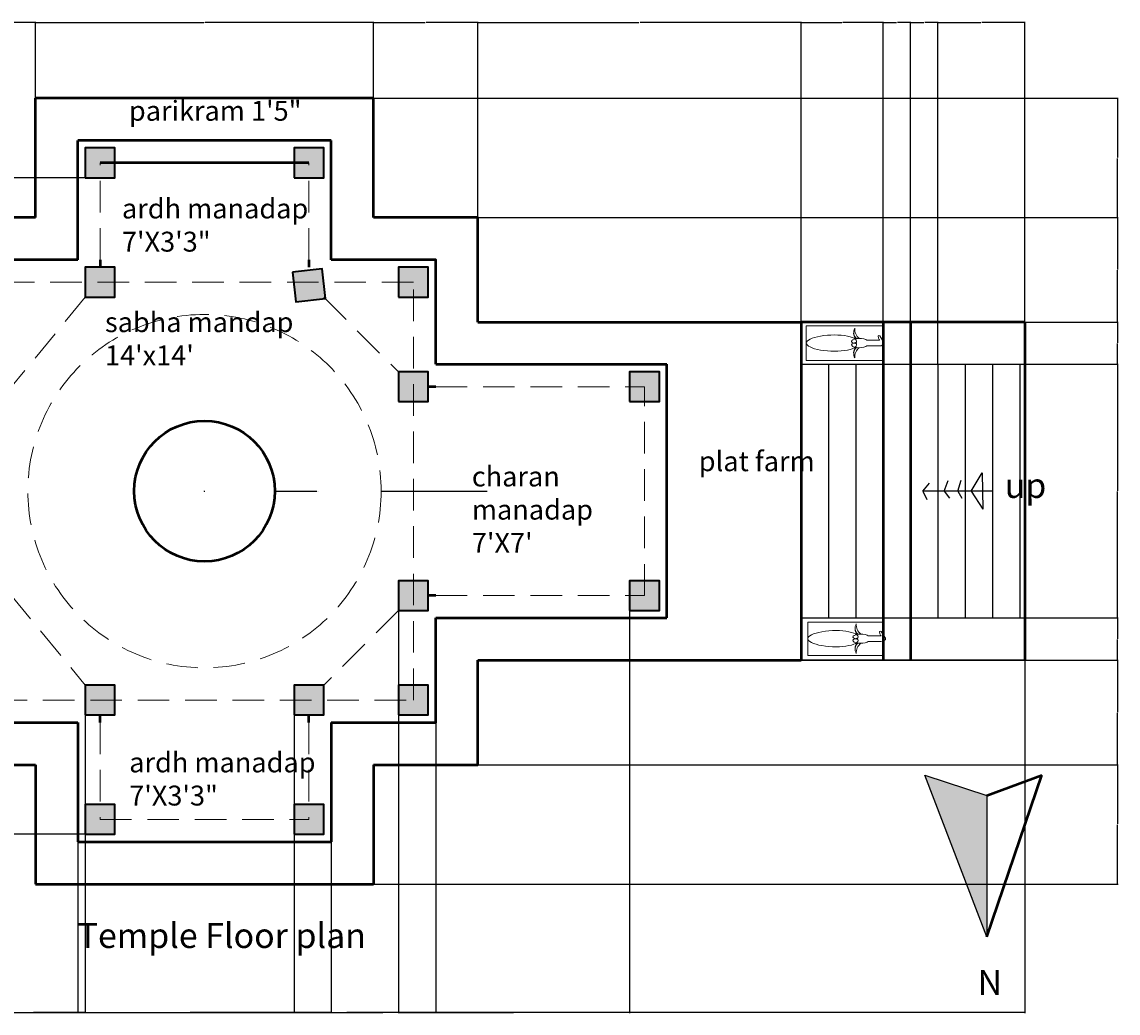
# Model space of a CAD drawing. Units: inches. Extents: x 386 to 107067, y -7 to 96314.
# Tile 6 of 10: x 766 to 1206, y 872 to 1271. Entities that reach past the tile are written whole.
import ezdxf

# ---------------------------------------------------------------- set-up
doc = ezdxf.new("R2010")
doc.units = ezdxf.units.IN
doc.linetypes.add('DASHED', pattern=[19.05, 12.7, -6.35])
for name, color, linetype, lineweight in [('A-ANNO-DIMS', 2, 'Continuous', 18), ('A-ANNO-SYMB', 2, 'Continuous', 25), ('A-ANNO-TEXT', 7, 'Continuous', 25), ('A-AREA-IDEN', 3, 'Continuous', 18), ('A-COLS', 1, 'Continuous', 35), ('A-FLOR-OVHD', 8, 'DASHED', 18), ('A-FLOR-STRS', 3, 'Continuous', 25), ('A-FURN', 8, 'Continuous', 18), ('A-WALL', 7, 'Continuous', 50)]:
    doc.layers.add(name, color=color, linetype=linetype, lineweight=lineweight)
doc.styles.get("Standard").update_dxf_attribs({"font": 'arial.ttf'})
doc.dimstyles.get("Standard").update_dxf_attribs({"dimtxt": 0.18, "dimasz": 0.18, "dimexe": 0.18, "dimexo": 0.0625, "dimgap": 0.09, "dimtad": 0, "dimtih": 1, "dimtoh": 1, "dimdec": 4, "dimzin": 0, "dimdsep": 46, "dimtxsty": 'Standard', "dimcen": 0.09, "dimadec": 0, "dimazin": 0, "dimtfac": 1, "dimtdec": 4, "dimtofl": 0, "dimtmove": 0, "dimatfit": 3, "dimfxl": 1, "dimtolj": 1, "dimtzin": 0, "dimarcsym": 0})

# ---------------------------------------------------------------- blocks, each defined once
blk = doc.blocks.new('COL-300')
h = blk.add_hatch(color=256)
h.dxf.hatch_style = 1
h.paths.add_polyline_path([(761.03, 1172.09), (749.03, 1172.09), (749.03, 1160.09), (761.03, 1160.09)])
blk.add_lwpolyline([(749.03, 1160.09), (761.03, 1160.09), (761.03, 1172.09), (749.03, 1172.09)], close=True)
blk = doc.blocks.new('*D8')
at = {"layer": 'A-ANNO-DIMS', "color": 0, "lineweight": -2, "transparency": 16777216}
for p, q in [((623.03, 1046.53), (623.03, 872.22)), ((1169.03, 1014.03), (1169.03, 872.22)), ((623.21, 872.4), (895.74, 872.4)), ((1168.85, 872.4), (896.31, 872.4))]:
    blk.add_line(p, q, dxfattribs=at)
at = {"layer": 'A-ANNO-DIMS', "color": 0, "transparency": 16777216}
for points in [[(623.21, 872.43), (623.21, 872.37), (623.03, 872.4)], [(1168.85, 872.43), (1168.85, 872.37), (1169.03, 872.4)]]:
    blk.add_solid(points, dxfattribs=at)
at = {"layer": 'Defpoints', "color": 0, "transparency": 16777216}
for p in [(623.03, 1046.59), (1169.03, 1014.09), (1169.03, 872.4)]:
    blk.add_point(p, dxfattribs=at)
at = {"layer": 'A-ANNO-DIMS', "color": 0, "transparency": 16777216, "insert": (896.03, 872.4), "char_height": 0.18, "attachment_point": 5}
blk.add_mtext('\\A1;546', dxfattribs=at)
blk = doc.blocks.new('*D10')
at = {"layer": 'A-ANNO-DIMS', "color": 0, "lineweight": -2, "transparency": 16777216}
for p, q in [((729.03, 1192.15), (729.03, 1270.77)), ((729.21, 1270.59), (749.8, 1270.59)), ((770.85, 1270.59), (750.25, 1270.59)), ((771.03, 1240.15), (771.03, 1270.77))]:
    blk.add_line(p, q, dxfattribs=at)
at = {"layer": 'A-ANNO-DIMS', "color": 0, "transparency": 16777216}
for points in [[(729.21, 1270.62), (729.21, 1270.56), (729.03, 1270.59)], [(770.85, 1270.62), (770.85, 1270.56), (771.03, 1270.59)]]:
    blk.add_solid(points, dxfattribs=at)
at = {"layer": 'Defpoints', "color": 0, "transparency": 16777216}
for p in [(771.03, 1270.59), (771.03, 1240.09), (729.03, 1192.09)]:
    blk.add_point(p, dxfattribs=at)
at = {"layer": 'A-ANNO-DIMS', "color": 0, "transparency": 16777216, "insert": (750.03, 1270.59), "char_height": 0.18, "attachment_point": 5}
blk.add_mtext('\\A1;42', dxfattribs=at)
blk = doc.blocks.new('*D11')
at = {"layer": 'A-ANNO-DIMS', "color": 0, "lineweight": -2, "transparency": 16777216}
for p, q in [((771.03, 1240.15), (771.03, 1270.77)), ((771.21, 1270.59), (838.74, 1270.59)), ((906.85, 1270.59), (839.31, 1270.59)), ((907.03, 1240.15), (907.03, 1270.77))]:
    blk.add_line(p, q, dxfattribs=at)
at = {"layer": 'A-ANNO-DIMS', "color": 0, "transparency": 16777216}
for points in [[(771.21, 1270.62), (771.21, 1270.56), (771.03, 1270.59)], [(906.85, 1270.62), (906.85, 1270.56), (907.03, 1270.59)]]:
    blk.add_solid(points, dxfattribs=at)
at = {"layer": 'Defpoints', "color": 0, "transparency": 16777216}
for p in [(907.03, 1270.59), (771.03, 1240.09), (907.03, 1240.09)]:
    blk.add_point(p, dxfattribs=at)
at = {"layer": 'A-ANNO-DIMS', "color": 0, "transparency": 16777216, "insert": (839.03, 1270.59), "char_height": 0.18, "attachment_point": 5}
blk.add_mtext('\\A1;136', dxfattribs=at)
blk = doc.blocks.new('*D12')
at = {"layer": 'A-ANNO-DIMS', "color": 0, "lineweight": -2, "transparency": 16777216}
for p, q in [((907.03, 1240.15), (907.03, 1270.77)), ((907.21, 1270.59), (927.8, 1270.59)), ((948.85, 1270.59), (928.25, 1270.59)), ((949.03, 1192.15), (949.03, 1270.77))]:
    blk.add_line(p, q, dxfattribs=at)
at = {"layer": 'A-ANNO-DIMS', "color": 0, "transparency": 16777216}
for points in [[(907.21, 1270.62), (907.21, 1270.56), (907.03, 1270.59)], [(948.85, 1270.62), (948.85, 1270.56), (949.03, 1270.59)]]:
    blk.add_solid(points, dxfattribs=at)
at = {"layer": 'Defpoints', "color": 0, "transparency": 16777216}
for p in [(949.03, 1270.59), (907.03, 1240.09), (949.03, 1192.09)]:
    blk.add_point(p, dxfattribs=at)
at = {"layer": 'A-ANNO-DIMS', "color": 0, "transparency": 16777216, "insert": (928.03, 1270.59), "char_height": 0.18, "attachment_point": 5}
blk.add_mtext('\\A1;42', dxfattribs=at)
blk = doc.blocks.new('*D13')
at = {"layer": 'A-ANNO-DIMS', "color": 0, "lineweight": -2, "transparency": 16777216}
for p, q in [((949.03, 1150.15), (949.03, 1270.77)), ((949.21, 1270.59), (1013.75, 1270.59)), ((1078.85, 1270.59), (1014.31, 1270.59)), ((1079.03, 1150.15), (1079.03, 1270.77))]:
    blk.add_line(p, q, dxfattribs=at)
at = {"layer": 'A-ANNO-DIMS', "color": 0, "transparency": 16777216}
for points in [[(949.21, 1270.62), (949.21, 1270.56), (949.03, 1270.59)], [(1078.85, 1270.62), (1078.85, 1270.56), (1079.03, 1270.59)]]:
    blk.add_solid(points, dxfattribs=at)
at = {"layer": 'Defpoints', "color": 0, "transparency": 16777216}
for p in [(1079.03, 1270.59), (949.03, 1150.09), (1079.03, 1150.09)]:
    blk.add_point(p, dxfattribs=at)
at = {"layer": 'A-ANNO-DIMS', "color": 0, "transparency": 16777216, "insert": (1014.03, 1270.59), "char_height": 0.18, "attachment_point": 5}
blk.add_mtext('\\A1;130', dxfattribs=at)
blk = doc.blocks.new('*D14')
at = {"layer": 'A-ANNO-DIMS', "color": 0, "lineweight": -2, "transparency": 16777216}
for p, q in [((1079.03, 1150.15), (1079.03, 1270.77)), ((1079.21, 1270.59), (1095.31, 1270.59)), ((1111.85, 1270.59), (1095.74, 1270.59)), ((1112.03, 1150.15), (1112.03, 1270.77))]:
    blk.add_line(p, q, dxfattribs=at)
at = {"layer": 'A-ANNO-DIMS', "color": 0, "transparency": 16777216}
for points in [[(1079.21, 1270.62), (1079.21, 1270.56), (1079.03, 1270.59)], [(1111.85, 1270.62), (1111.85, 1270.56), (1112.03, 1270.59)]]:
    blk.add_solid(points, dxfattribs=at)
at = {"layer": 'Defpoints', "color": 0, "transparency": 16777216}
for p in [(1112.03, 1270.59), (1079.03, 1150.09), (1112.03, 1150.09)]:
    blk.add_point(p, dxfattribs=at)
at = {"layer": 'A-ANNO-DIMS', "color": 0, "transparency": 16777216, "insert": (1095.53, 1270.59), "char_height": 0.18, "attachment_point": 5}
blk.add_mtext('\\A1;33', dxfattribs=at)
blk = doc.blocks.new('*D15')
at = {"layer": 'A-ANNO-DIMS', "color": 0, "lineweight": -2, "transparency": 16777216}
for p, q in [((1112.03, 1150.15), (1112.03, 1270.77)), ((1112.21, 1270.59), (1117.33, 1270.59)), ((1122.85, 1270.59), (1117.72, 1270.59)), ((1123.03, 1150.15), (1123.03, 1270.77))]:
    blk.add_line(p, q, dxfattribs=at)
at = {"layer": 'A-ANNO-DIMS', "color": 0, "transparency": 16777216}
for points in [[(1112.21, 1270.62), (1112.21, 1270.56), (1112.03, 1270.59)], [(1122.85, 1270.62), (1122.85, 1270.56), (1123.03, 1270.59)]]:
    blk.add_solid(points, dxfattribs=at)
at = {"layer": 'Defpoints', "color": 0, "transparency": 16777216}
for p in [(1123.03, 1270.59), (1112.03, 1150.09), (1123.03, 1150.09)]:
    blk.add_point(p, dxfattribs=at)
at = {"layer": 'A-ANNO-DIMS', "color": 0, "transparency": 16777216, "insert": (1117.53, 1270.59), "char_height": 0.18, "attachment_point": 5}
blk.add_mtext('\\A1;11', dxfattribs=at)
blk = doc.blocks.new('*D16')
at = {"layer": 'A-ANNO-DIMS', "color": 0, "lineweight": -2, "transparency": 16777216}
for p, q in [((1123.03, 1150.15), (1123.03, 1270.77)), ((1123.21, 1270.59), (1128.33, 1270.59)), ((1133.85, 1270.59), (1128.72, 1270.59)), ((1134.03, 1133.15), (1134.03, 1270.77))]:
    blk.add_line(p, q, dxfattribs=at)
at = {"layer": 'A-ANNO-DIMS', "color": 0, "transparency": 16777216}
for points in [[(1123.21, 1270.62), (1123.21, 1270.56), (1123.03, 1270.59)], [(1133.85, 1270.62), (1133.85, 1270.56), (1134.03, 1270.59)]]:
    blk.add_solid(points, dxfattribs=at)
at = {"layer": 'Defpoints', "color": 0, "transparency": 16777216}
for p in [(1134.03, 1270.59), (1123.03, 1150.09), (1134.03, 1133.09)]:
    blk.add_point(p, dxfattribs=at)
at = {"layer": 'A-ANNO-DIMS', "color": 0, "transparency": 16777216, "insert": (1128.53, 1270.59), "char_height": 0.18, "attachment_point": 5}
blk.add_mtext('\\A1;11', dxfattribs=at)
blk = doc.blocks.new('*D17')
at = {"layer": 'A-ANNO-DIMS', "color": 0, "lineweight": -2, "transparency": 16777216}
for p, q in [((1134.03, 1133.15), (1134.03, 1270.77)), ((1134.21, 1270.59), (1151.31, 1270.59)), ((1168.85, 1270.59), (1151.74, 1270.59)), ((1169.03, 1150.15), (1169.03, 1270.77))]:
    blk.add_line(p, q, dxfattribs=at)
at = {"layer": 'A-ANNO-DIMS', "color": 0, "transparency": 16777216}
for points in [[(1134.21, 1270.62), (1134.21, 1270.56), (1134.03, 1270.59)], [(1168.85, 1270.62), (1168.85, 1270.56), (1169.03, 1270.59)]]:
    blk.add_solid(points, dxfattribs=at)
at = {"layer": 'Defpoints', "color": 0, "transparency": 16777216}
for p in [(1169.03, 1270.59), (1169.03, 1150.09), (1134.03, 1133.09)]:
    blk.add_point(p, dxfattribs=at)
at = {"layer": 'A-ANNO-DIMS', "color": 0, "transparency": 16777216, "insert": (1151.53, 1270.59), "char_height": 0.18, "attachment_point": 5}
blk.add_mtext('\\A1;35', dxfattribs=at)
blk = doc.blocks.new('*D18')
at = {"layer": 'A-ANNO-DIMS', "color": 0, "lineweight": -2, "transparency": 16777216}
for p, q in [((949.09, 972.09), (1206.45, 972.09)), ((1206.27, 971.91), (1206.27, 948.27)), ((1206.27, 924.27), (1206.27, 947.91)), ((907.09, 924.09), (1206.45, 924.09))]:
    blk.add_line(p, q, dxfattribs=at)
at = {"layer": 'A-ANNO-DIMS', "color": 0, "transparency": 16777216}
for points in [[(1206.24, 971.91), (1206.3, 971.91), (1206.27, 972.09)], [(1206.24, 924.27), (1206.3, 924.27), (1206.27, 924.09)]]:
    blk.add_solid(points, dxfattribs=at)
at = {"layer": 'Defpoints', "color": 0, "transparency": 16777216}
for p in [(949.03, 972.09), (1206.27, 972.09), (907.03, 924.09)]:
    blk.add_point(p, dxfattribs=at)
at = {"layer": 'A-ANNO-DIMS', "color": 0, "transparency": 16777216, "insert": (1206.27, 948.09), "char_height": 0.18, "attachment_point": 5}
blk.add_mtext('\\A1;48', dxfattribs=at)
blk = doc.blocks.new('*D19')
at = {"layer": 'A-ANNO-DIMS', "color": 0, "lineweight": -2, "transparency": 16777216}
for p, q in [((1079.09, 1014.09), (1206.45, 1014.09)), ((1206.27, 1013.91), (1206.27, 993.27)), ((1206.27, 972.27), (1206.27, 992.91)), ((949.09, 972.09), (1206.45, 972.09))]:
    blk.add_line(p, q, dxfattribs=at)
at = {"layer": 'A-ANNO-DIMS', "color": 0, "transparency": 16777216}
for points in [[(1206.24, 1013.91), (1206.3, 1013.91), (1206.27, 1014.09)], [(1206.24, 972.27), (1206.3, 972.27), (1206.27, 972.09)]]:
    blk.add_solid(points, dxfattribs=at)
at = {"layer": 'Defpoints', "color": 0, "transparency": 16777216}
for p in [(1079.03, 1014.09), (1206.27, 1014.09), (949.03, 972.09)]:
    blk.add_point(p, dxfattribs=at)
at = {"layer": 'A-ANNO-DIMS', "color": 0, "transparency": 16777216, "insert": (1206.27, 993.09), "char_height": 0.18, "attachment_point": 5}
blk.add_mtext('\\A1;42', dxfattribs=at)
blk = doc.blocks.new('*D20')
at = {"layer": 'A-ANNO-DIMS', "color": 0, "lineweight": -2, "transparency": 16777216}
for p, q in [((1169.09, 1031.09), (1206.45, 1031.09)), ((1206.27, 1030.91), (1206.27, 1022.77)), ((1206.27, 1014.27), (1206.27, 1022.41)), ((1079.09, 1014.09), (1206.45, 1014.09))]:
    blk.add_line(p, q, dxfattribs=at)
at = {"layer": 'A-ANNO-DIMS', "color": 0, "transparency": 16777216}
for points in [[(1206.24, 1030.91), (1206.3, 1030.91), (1206.27, 1031.09)], [(1206.24, 1014.27), (1206.3, 1014.27), (1206.27, 1014.09)]]:
    blk.add_solid(points, dxfattribs=at)
at = {"layer": 'Defpoints', "color": 0, "transparency": 16777216}
for p in [(1169.03, 1031.09), (1206.27, 1031.09), (1079.03, 1014.09)]:
    blk.add_point(p, dxfattribs=at)
at = {"layer": 'A-ANNO-DIMS', "color": 0, "transparency": 16777216, "insert": (1206.27, 1022.59), "char_height": 0.18, "attachment_point": 5}
blk.add_mtext('\\A1;17', dxfattribs=at)
blk = doc.blocks.new('*D21')
at = {"layer": 'A-ANNO-DIMS', "color": 0, "lineweight": -2, "transparency": 16777216}
for p, q in [((1169.09, 1133.09), (1206.45, 1133.09)), ((1206.27, 1132.91), (1206.27, 1082.27)), ((1206.27, 1031.27), (1206.27, 1081.91)), ((1169.09, 1031.09), (1206.45, 1031.09))]:
    blk.add_line(p, q, dxfattribs=at)
at = {"layer": 'A-ANNO-DIMS', "color": 0, "transparency": 16777216}
for points in [[(1206.24, 1132.91), (1206.3, 1132.91), (1206.27, 1133.09)], [(1206.24, 1031.27), (1206.3, 1031.27), (1206.27, 1031.09)]]:
    blk.add_solid(points, dxfattribs=at)
at = {"layer": 'Defpoints', "color": 0, "transparency": 16777216}
for p in [(1169.03, 1133.09), (1206.27, 1133.09), (1169.03, 1031.09)]:
    blk.add_point(p, dxfattribs=at)
at = {"layer": 'A-ANNO-DIMS', "color": 0, "transparency": 16777216, "insert": (1206.27, 1082.09), "char_height": 0.18, "attachment_point": 5}
blk.add_mtext('\\A1;102', dxfattribs=at)
blk = doc.blocks.new('*D22')
at = {"layer": 'A-ANNO-DIMS', "color": 0, "lineweight": -2, "transparency": 16777216}
for p, q in [((1079.09, 1150.09), (1206.45, 1150.09)), ((1206.27, 1149.91), (1206.27, 1141.77)), ((1206.27, 1133.27), (1206.27, 1141.41)), ((1169.09, 1133.09), (1206.45, 1133.09))]:
    blk.add_line(p, q, dxfattribs=at)
at = {"layer": 'A-ANNO-DIMS', "color": 0, "transparency": 16777216}
for points in [[(1206.24, 1149.91), (1206.3, 1149.91), (1206.27, 1150.09)], [(1206.24, 1133.27), (1206.3, 1133.27), (1206.27, 1133.09)]]:
    blk.add_solid(points, dxfattribs=at)
at = {"layer": 'Defpoints', "color": 0, "transparency": 16777216}
for p in [(1079.03, 1150.09), (1206.27, 1150.09), (1169.03, 1133.09)]:
    blk.add_point(p, dxfattribs=at)
at = {"layer": 'A-ANNO-DIMS', "color": 0, "transparency": 16777216, "insert": (1206.27, 1141.59), "char_height": 0.18, "attachment_point": 5}
blk.add_mtext('\\A1;17', dxfattribs=at)
blk = doc.blocks.new('*D23')
at = {"layer": 'A-ANNO-DIMS', "color": 0, "lineweight": -2, "transparency": 16777216}
for p, q in [((949.09, 1192.09), (1206.45, 1192.09)), ((1206.27, 1191.91), (1206.27, 1171.27)), ((1206.27, 1150.27), (1206.27, 1170.91)), ((949.09, 1150.09), (1206.45, 1150.09))]:
    blk.add_line(p, q, dxfattribs=at)
at = {"layer": 'A-ANNO-DIMS', "color": 0, "transparency": 16777216}
for points in [[(1206.24, 1191.91), (1206.3, 1191.91), (1206.27, 1192.09)], [(1206.24, 1150.27), (1206.3, 1150.27), (1206.27, 1150.09)]]:
    blk.add_solid(points, dxfattribs=at)
at = {"layer": 'Defpoints', "color": 0, "transparency": 16777216}
for p in [(949.03, 1192.09), (1206.27, 1192.09), (949.03, 1150.09)]:
    blk.add_point(p, dxfattribs=at)
at = {"layer": 'A-ANNO-DIMS', "color": 0, "transparency": 16777216, "insert": (1206.27, 1171.09), "char_height": 0.18, "attachment_point": 5}
blk.add_mtext('\\A1;42', dxfattribs=at)
blk = doc.blocks.new('*D24')
at = {"layer": 'A-ANNO-DIMS', "color": 0, "lineweight": -2, "transparency": 16777216}
for p, q in [((907.09, 1240.09), (1206.45, 1240.09)), ((1206.27, 1239.91), (1206.27, 1216.27)), ((1206.27, 1192.27), (1206.27, 1215.91)), ((907.09, 1192.09), (1206.45, 1192.09))]:
    blk.add_line(p, q, dxfattribs=at)
at = {"layer": 'A-ANNO-DIMS', "color": 0, "transparency": 16777216}
for points in [[(1206.24, 1239.91), (1206.3, 1239.91), (1206.27, 1240.09)], [(1206.24, 1192.27), (1206.3, 1192.27), (1206.27, 1192.09)]]:
    blk.add_solid(points, dxfattribs=at)
at = {"layer": 'Defpoints', "color": 0, "transparency": 16777216}
for p in [(907.03, 1240.09), (1206.27, 1240.09), (907.03, 1192.09)]:
    blk.add_point(p, dxfattribs=at)
at = {"layer": 'A-ANNO-DIMS', "color": 0, "transparency": 16777216, "insert": (1206.27, 1216.09), "char_height": 0.18, "attachment_point": 5}
blk.add_mtext('\\A1;48', dxfattribs=at)
blk = doc.blocks.new('*D25')
at = {"layer": 'A-ANNO-DIMS', "color": 0, "lineweight": -2, "transparency": 16777216}
for p, q in [((788.03, 941.03), (788.03, 872.22)), ((890.03, 941.03), (890.03, 872.22)), ((788.21, 872.4), (838.75, 872.4)), ((889.85, 872.4), (839.3, 872.4))]:
    blk.add_line(p, q, dxfattribs=at)
at = {"layer": 'A-ANNO-DIMS', "color": 0, "transparency": 16777216}
for points in [[(788.21, 872.43), (788.21, 872.37), (788.03, 872.4)], [(889.85, 872.43), (889.85, 872.37), (890.03, 872.4)]]:
    blk.add_solid(points, dxfattribs=at)
at = {"layer": 'Defpoints', "color": 0, "transparency": 16777216}
for p in [(788.03, 941.09), (890.03, 941.09), (890.03, 872.4)]:
    blk.add_point(p, dxfattribs=at)
at = {"layer": 'A-ANNO-DIMS', "color": 0, "transparency": 16777216, "insert": (839.03, 872.4), "char_height": 0.18, "attachment_point": 5}
blk.add_mtext('\\A1;102', dxfattribs=at)
blk = doc.blocks.new('*D26')
at = {"layer": 'A-ANNO-DIMS', "color": 0, "lineweight": -2, "transparency": 16777216}
for p, q in [((932.03, 989.03), (932.03, 872.22)), ((890.03, 941.03), (890.03, 872.22)), ((890.21, 872.4), (910.8, 872.4)), ((931.85, 872.4), (911.25, 872.4))]:
    blk.add_line(p, q, dxfattribs=at)
at = {"layer": 'A-ANNO-DIMS', "color": 0, "transparency": 16777216}
for points in [[(890.21, 872.43), (890.21, 872.37), (890.03, 872.4)], [(931.85, 872.43), (931.85, 872.37), (932.03, 872.4)]]:
    blk.add_solid(points, dxfattribs=at)
at = {"layer": 'Defpoints', "color": 0, "transparency": 16777216}
for p in [(932.03, 989.09), (890.03, 941.09), (932.03, 872.4)]:
    blk.add_point(p, dxfattribs=at)
at = {"layer": 'A-ANNO-DIMS', "color": 0, "transparency": 16777216, "insert": (911.03, 872.4), "char_height": 0.18, "attachment_point": 5}
blk.add_mtext('\\A1;42', dxfattribs=at)
blk = doc.blocks.new('*D27')
at = {"layer": 'A-ANNO-DIMS', "color": 0, "lineweight": -2, "transparency": 16777216}
for p, q in [((749.03, 992.03), (749.03, 872.22)), ((791.03, 992.03), (791.03, 872.22)), ((749.21, 872.4), (769.8, 872.4)), ((790.85, 872.4), (770.25, 872.4))]:
    blk.add_line(p, q, dxfattribs=at)
at = {"layer": 'A-ANNO-DIMS', "color": 0, "transparency": 16777216}
for points in [[(749.21, 872.43), (749.21, 872.37), (749.03, 872.4)], [(790.85, 872.43), (790.85, 872.37), (791.03, 872.4)]]:
    blk.add_solid(points, dxfattribs=at)
at = {"layer": 'Defpoints', "color": 0, "transparency": 16777216}
for p in [(749.03, 992.09), (791.03, 992.09), (791.03, 872.4)]:
    blk.add_point(p, dxfattribs=at)
at = {"layer": 'A-ANNO-DIMS', "color": 0, "transparency": 16777216, "insert": (770.03, 872.4), "char_height": 0.18, "attachment_point": 5}
blk.add_mtext('\\A1;42', dxfattribs=at)
blk = doc.blocks.new('*D28')
at = {"layer": 'A-ANNO-DIMS', "color": 0, "lineweight": -2, "transparency": 16777216}
for p, q in [((791.03, 992.03), (791.03, 872.22)), ((875.03, 992.03), (875.03, 872.22)), ((791.21, 872.4), (832.81, 872.4)), ((874.85, 872.4), (833.24, 872.4))]:
    blk.add_line(p, q, dxfattribs=at)
at = {"layer": 'A-ANNO-DIMS', "color": 0, "transparency": 16777216}
for points in [[(791.21, 872.43), (791.21, 872.37), (791.03, 872.4)], [(874.85, 872.43), (874.85, 872.37), (875.03, 872.4)]]:
    blk.add_solid(points, dxfattribs=at)
at = {"layer": 'Defpoints', "color": 0, "transparency": 16777216}
for p in [(791.03, 992.09), (875.03, 992.09), (875.03, 872.4)]:
    blk.add_point(p, dxfattribs=at)
at = {"layer": 'A-ANNO-DIMS', "color": 0, "transparency": 16777216, "insert": (833.03, 872.4), "char_height": 0.18, "attachment_point": 5}
blk.add_mtext('\\A1;84', dxfattribs=at)
blk = doc.blocks.new('*D29')
at = {"layer": 'A-ANNO-DIMS', "color": 0, "lineweight": -2, "transparency": 16777216}
for p, q in [((875.03, 992.03), (875.03, 872.22)), ((917.03, 992.03), (917.03, 872.22)), ((875.21, 872.4), (895.8, 872.4)), ((916.85, 872.4), (896.25, 872.4))]:
    blk.add_line(p, q, dxfattribs=at)
at = {"layer": 'A-ANNO-DIMS', "color": 0, "transparency": 16777216}
for points in [[(875.21, 872.43), (875.21, 872.37), (875.03, 872.4)], [(916.85, 872.43), (916.85, 872.37), (917.03, 872.4)]]:
    blk.add_solid(points, dxfattribs=at)
at = {"layer": 'Defpoints', "color": 0, "transparency": 16777216}
for p in [(875.03, 992.09), (917.03, 992.09), (917.03, 872.4)]:
    blk.add_point(p, dxfattribs=at)
at = {"layer": 'A-ANNO-DIMS', "color": 0, "transparency": 16777216, "insert": (896.03, 872.4), "char_height": 0.18, "attachment_point": 5}
blk.add_mtext('\\A1;42', dxfattribs=at)
blk = doc.blocks.new('*D30')
at = {"layer": 'A-ANNO-DIMS', "color": 0, "lineweight": -2, "transparency": 16777216}
for p, q in [((917.03, 1034.03), (917.03, 872.22)), ((1010.03, 1034.03), (1010.03, 872.22)), ((917.21, 872.4), (963.31, 872.4)), ((1009.85, 872.4), (963.74, 872.4))]:
    blk.add_line(p, q, dxfattribs=at)
at = {"layer": 'A-ANNO-DIMS', "color": 0, "transparency": 16777216}
for points in [[(917.21, 872.43), (917.21, 872.37), (917.03, 872.4)], [(1009.85, 872.43), (1009.85, 872.37), (1010.03, 872.4)]]:
    blk.add_solid(points, dxfattribs=at)
at = {"layer": 'Defpoints', "color": 0, "transparency": 16777216}
for p in [(917.03, 1034.09), (1010.03, 1034.09), (1010.03, 872.4)]:
    blk.add_point(p, dxfattribs=at)
at = {"layer": 'A-ANNO-DIMS', "color": 0, "transparency": 16777216, "insert": (963.53, 872.4), "char_height": 0.18, "attachment_point": 5}
blk.add_mtext('\\A1;93', dxfattribs=at)
blk = doc.blocks.new('*D31')
at = {"layer": 'A-ANNO-DIMS', "color": 0, "lineweight": -2, "transparency": 16777216}
for p, q in [((748.96, 992.09), (592.35, 992.09)), ((592.53, 991.91), (592.53, 968.27)), ((592.53, 944.27), (592.53, 967.91)), ((790.96, 944.09), (592.35, 944.09))]:
    blk.add_line(p, q, dxfattribs=at)
at = {"layer": 'A-ANNO-DIMS', "color": 0, "transparency": 16777216}
for points in [[(592.5, 991.91), (592.56, 991.91), (592.53, 992.09)], [(592.5, 944.27), (592.56, 944.27), (592.53, 944.09)]]:
    blk.add_solid(points, dxfattribs=at)
at = {"layer": 'Defpoints', "color": 0, "transparency": 16777216}
for p in [(592.53, 992.09), (749.03, 992.09), (791.03, 944.09)]:
    blk.add_point(p, dxfattribs=at)
at = {"layer": 'A-ANNO-DIMS', "color": 0, "transparency": 16777216, "insert": (592.53, 968.09), "char_height": 0.18, "attachment_point": 5}
blk.add_mtext('\\A1;48', dxfattribs=at)
blk = doc.blocks.new('*D35')
at = {"layer": 'A-ANNO-DIMS', "color": 0, "lineweight": -2, "transparency": 16777216}
for p, q in [((790.96, 1208.09), (592.35, 1208.09)), ((592.53, 1207.91), (592.53, 1184.27)), ((592.53, 1160.27), (592.53, 1183.91)), ((748.96, 1160.09), (592.35, 1160.09))]:
    blk.add_line(p, q, dxfattribs=at)
at = {"layer": 'A-ANNO-DIMS', "color": 0, "transparency": 16777216}
for points in [[(592.5, 1207.91), (592.56, 1207.91), (592.53, 1208.09)], [(592.5, 1160.27), (592.56, 1160.27), (592.53, 1160.09)]]:
    blk.add_solid(points, dxfattribs=at)
at = {"layer": 'Defpoints', "color": 0, "transparency": 16777216}
for p in [(592.53, 1208.09), (791.03, 1208.09), (749.03, 1160.09)]:
    blk.add_point(p, dxfattribs=at)
at = {"layer": 'A-ANNO-DIMS', "color": 0, "transparency": 16777216, "insert": (592.53, 1184.09), "char_height": 0.18, "attachment_point": 5}
blk.add_mtext('\\A1;48', dxfattribs=at)
blk = doc.blocks.new('*D85')
at = {"layer": 'A-ANNO-DIMS', "color": 0, "lineweight": -2, "transparency": 16777216}
for p, q in [((838.94, 1082.09), (839.12, 1082.09)), ((839.03, 1082), (839.03, 1082.18)), ((952.7, 1081.94), (910.25, 1082))]:
    blk.add_line(p, q, dxfattribs=at)
at = {"layer": 'A-ANNO-DIMS', "color": 0, "transparency": 16777216}
blk.add_solid([(910.25, 1082.03), (910.25, 1081.97), (910.07, 1082)], dxfattribs=at)
at = {"layer": 'Defpoints', "color": 0, "transparency": 16777216}
for p in [(767.98, 1082.18), (910.07, 1082)]:
    blk.add_point(p, dxfattribs=at)
at = {"layer": 'A-ANNO-DIMS', "color": 0, "transparency": 16777216, "insert": (953.18, 1081.94), "char_height": 0.18, "attachment_point": 5}
blk.add_mtext('\\A1;∅142.1', dxfattribs=at)
blk = doc.blocks.new('*D86')
at = {"layer": 'A-ANNO-DIMS', "color": 0, "lineweight": -2, "transparency": 16777216}
for p, q in [((838.94, 1082.09), (839.12, 1082.09)), ((839.03, 1082), (839.03, 1082.18)), ((884.26, 1081.94), (867.47, 1082))]:
    blk.add_line(p, q, dxfattribs=at)
at = {"layer": 'A-ANNO-DIMS', "color": 0, "transparency": 16777216}
blk.add_solid([(867.47, 1082.03), (867.47, 1081.97), (867.29, 1082)], dxfattribs=at)
at = {"layer": 'Defpoints', "color": 0, "transparency": 16777216}
for p in [(810.76, 1082.18), (867.29, 1082)]:
    blk.add_point(p, dxfattribs=at)
at = {"layer": 'A-ANNO-DIMS', "color": 0, "transparency": 16777216, "insert": (884.75, 1081.94), "char_height": 0.18, "attachment_point": 5}
blk.add_mtext('\\A1;∅56.54', dxfattribs=at)

msp = doc.modelspace()

# ---------------------------------------------------------------- hatches: boundary and pattern name
at = {"layer": 'A-ANNO-SYMB'}
h = msp.add_hatch(color=256, dxfattribs=at)
h.dxf.hatch_style = 1
h.paths.add_polyline_path([(1153.7023, 959.756), (1128.7329, 967.879), (1153.7023, 902.8951)])

# ---------------------------------------------------------------- linework, layer by layer
for p, q in [((1153.7023, 902.8951), (1128.7329, 967.879)), ((1128.7329, 967.879), (1153.7023, 959.756)), ((1153.7023, 959.756), (1153.7023, 902.8951))]:
    msp.add_line(p, q, dxfattribs=at)
at = {"layer": 'A-FLOR-OVHD'}
for p, q in [((797.0252, 1175.0919), (797.0252, 1214.0919)), ((881.0252, 1175.0919), (881.0252, 1214.0919)), ((791.0252, 1160.0919), (761.0252, 1123.5919)), ((887.0252, 1160.0919), (917.0252, 1130.0919)), ((932.0252, 1124.0919), (1016.0252, 1124.0919)), ((761.0252, 1040.5919), (791.0252, 1004.0919)), ((932.0252, 1040.0919), (1016.0252, 1040.0919)), ((917.0252, 1034.0919), (887.0252, 1004.0919)), ((797.0252, 989.0919), (797.0252, 950.0919)), ((881.0252, 989.0919), (881.0252, 950.0919))]:
    msp.add_line(p, q, dxfattribs=at)
msp.add_lwpolyline([(755.0252, 998.0919), (923.0252, 998.0919), (923.0252, 1166.0919), (755.0252, 1166.0919)], close=True, dxfattribs=at)
for points in [[(1016.0252, 1040.0919), (1016.0252, 1124.0919)], [(797.0252, 950.0919), (881.0252, 950.0919)]]:
    msp.add_lwpolyline(points, dxfattribs=at)
msp.add_circle((839.0252, 1082.0919), 71.0489, dxfattribs=at)
at = {"layer": 'A-FLOR-STRS'}
for p, q in [((1079.0252, 1133.0919), (1169.0252, 1133.0919)), ((1090.0252, 1133.0919), (1090.0252, 1031.0919)), ((1101.0252, 1133.0919), (1101.0252, 1031.0919)), ((1134.0252, 1133.0919), (1134.0252, 1031.0919)), ((1145.0252, 1133.0919), (1145.0252, 1031.0919)), ((1156.0252, 1133.0919), (1156.0252, 1031.0919)), ((1167.0252, 1133.0919), (1167.0252, 1031.0919)), ((1147.3807, 1082.0919), (1151.8475, 1089.4417)), ((1151.8475, 1089.4417), (1152.0507, 1074.8695)), ((1127.9633, 1082.0919), (1130.6308, 1085.3314)), ((1136.5839, 1082.0919), (1138.1948, 1086.3111)), ((1141.9943, 1082.0919), (1143.3605, 1086.5406)), ((1156.0252, 1082.0919), (1127.9633, 1082.0919)), ((1127.9633, 1082.0919), (1129.5103, 1078.6833)), ((1136.5839, 1082.0919), (1138.615, 1079.2431)), ((1141.9943, 1082.0919), (1143.6576, 1079.3131)), ((1147.3807, 1082.0919), (1152.0507, 1074.8695)), ((1079.0252, 1031.0919), (1169.0252, 1031.0919)), ((1169.0252, 1014.0919), (1079.0252, 1014.0919))]:
    msp.add_line(p, q, dxfattribs=at)
at = {"layer": 'A-FURN'}
for p, q in [((1105.4478, 1142.7372), (1110.5041, 1142.7946)), ((1110.0845, 1143.5893), (1109.9557, 1144.4901)), ((1110.6313, 1144.5352), (1112.3255, 1141.8164)), ((1105.4478, 1140.5249), (1110.5041, 1140.4675)), ((1106.0067, 1023.8699), (1111.063, 1023.9273)), ((1110.6434, 1024.722), (1110.5146, 1025.6228)), ((1111.1902, 1025.6679), (1112.8845, 1022.9491)), ((1106.0067, 1021.6576), (1111.063, 1021.6002))]:
    msp.add_line(p, q, dxfattribs=at)
for points in [[(1081.0679, 1148.506), (1112.0252, 1148.506), (1112.0252, 1134.6088), (1081.0679, 1134.6088)], [(1081.6268, 1029.418), (1112.0252, 1029.418), (1112.0252, 1015.9622), (1081.6268, 1015.9622)]]:
    msp.add_lwpolyline(points, close=True, dxfattribs=at)
for centre, radius, start, end in [((1104.0477, 1145.6688), 3.9284, 150.303849, 216.308119), ((1103.6019, 1145.8978), 3.4278, 149.936449, 226.630675), ((1105.0545, 1147.1), 4.4492, 173.353928, 234.224432), ((1104.0477, 1137.5934), 3.9284, 143.691881, 209.696151), ((1103.6019, 1137.3644), 3.4278, 133.369325, 210.063551), ((1105.0545, 1136.1621), 4.4492, 125.775568, 186.646072), ((1104.6067, 1026.8015), 3.9284, 150.303849, 216.308119), ((1104.1608, 1027.0305), 3.4278, 149.936449, 226.630675), ((1105.6135, 1028.2327), 4.4492, 173.353928, 234.224432), ((1104.6067, 1018.7261), 3.9284, 143.691881, 209.696151), ((1104.1608, 1018.4971), 3.4278, 133.369325, 210.063551), ((1105.6135, 1017.2948), 4.4492, 125.775568, 186.646072)]:
    msp.add_arc(centre, radius, start, end, dxfattribs=at)
for centre, major_axis, ratio, start_param, end_param in [((1091.1989, 1141.9468), (10.131, 0.3893), 0.28888768, 6.018681, 9.42477796), ((1102.4535, 1142.3663), (-3.172, 0), 0.35436306, 3.47793685, 7.32452327), ((1091.7578, 1023.0795), (10.131, 0.3893), 0.28888768, 6.018681, 9.42477796), ((1103.0124, 1023.499), (-3.172, 0), 0.35436306, 3.47793685, 7.32452327)]:
    msp.add_ellipse(centre, major_axis=major_axis, ratio=ratio, start_param=start_param, end_param=end_param, dxfattribs=at)
at = {"layer": 'A-FURN', "extrusion": (0, 0, -1)}
for centre, major_axis, ratio, start_param, end_param in [((1102.4535, 1140.8959), (-3.172, 0), 0.35436306, 3.47793685, 7.32452327), ((1091.1989, 1141.3154), (10.131, -0.3893), 0.28888768, 6.018681, 9.42477796), ((1091.7578, 1022.4481), (10.131, -0.3893), 0.28888768, 6.018681, 9.42477796), ((1103.0124, 1022.0286), (-3.172, 0), 0.35436306, 3.47793685, 7.32452327)]:
    msp.add_ellipse(centre, major_axis=major_axis, ratio=ratio, start_param=start_param, end_param=end_param, dxfattribs=at)
at = {"layer": 'A-FURN'}
for points in [[(1109.9557, 1144.4901), (1109.9237, 1144.7136), (1110.5119, 1144.7268), (1110.6313, 1144.5352)], [(1110.5041, 1142.7946), (1110.8036, 1142.798), (1110.1269, 1143.2928), (1110.0845, 1143.5893)], [(1110.5041, 1140.4675), (1111.2595, 1140.4589), (1112.7251, 1141.1752), (1112.3255, 1141.8164)], [(1110.5146, 1025.6228), (1110.4827, 1025.8463), (1111.0709, 1025.8595), (1111.1902, 1025.6679)], [(1111.063, 1023.9273), (1111.3625, 1023.9307), (1110.6858, 1024.4255), (1110.6434, 1024.722)], [(1111.063, 1021.6002), (1111.8185, 1021.5916), (1113.284, 1022.3079), (1112.8845, 1022.9491)]]:
    msp.add_open_spline(points, degree=3, dxfattribs=at)
at = {"layer": 'A-WALL'}
for p, q in [((771.0252, 1192.0919), (771.0252, 1240.0919)), ((907.0252, 1192.0919), (907.0252, 1240.0919)), ((788.0252, 1175.0919), (788.0252, 1223.0919)), ((890.0252, 1175.0919), (890.0252, 1223.0919)), ((797.0252, 1175.0919), (797.0252, 1172.0919)), ((881.0252, 1175.0919), (881.0252, 1172.0919)), ((949.0252, 1150.0919), (1079.0252, 1150.0919)), ((1079.0252, 1150.0919), (1079.0252, 1014.0919)), ((1169.0252, 1150.0919), (1079.0252, 1150.0919)), ((1112.0252, 1150.0919), (1112.0252, 1014.0919)), ((1123.0252, 1150.0919), (1123.0252, 1014.0919)), ((1169.0252, 1150.0919), (1169.0252, 1014.0919)), ((932.0252, 1133.0919), (1025.0252, 1133.0919)), ((932.0252, 1124.0919), (929.0252, 1124.0919)), ((932.0252, 1040.0919), (929.0252, 1040.0919)), ((932.0252, 1031.0919), (1025.0252, 1031.0919)), ((949.0252, 1014.0919), (1079.0252, 1014.0919)), ((797.0252, 989.0919), (797.0252, 992.0919)), ((881.0252, 989.0919), (881.0252, 992.0919)), ((788.0252, 989.0919), (788.0252, 941.0919)), ((890.0252, 989.0919), (890.0252, 941.0919)), ((771.0252, 972.0919), (771.0252, 924.0919)), ((907.0252, 972.0919), (907.0252, 924.0919)), ((1153.7023, 902.8951), (1175.7683, 967.879)), ((1153.7023, 959.756), (1175.7683, 967.879))]:
    msp.add_line(p, q, dxfattribs=at)
for points in [[(907.0252, 1240.0919), (771.0252, 1240.0919)], [(890.0252, 1223.0919), (788.0252, 1223.0919)], [(881.0252, 1214.0919), (797.0252, 1214.0919)], [(771.0252, 1192.0919), (729.0252, 1192.0919), (729.0252, 1152.5919)], [(949.0252, 1150.0919), (949.0252, 1192.0919), (907.0252, 1192.0919)], [(788.0252, 1175.0919), (746.0252, 1175.0919), (746.0252, 989.0919), (788.0252, 989.0919)], [(932.0252, 1133.0919), (932.0252, 1175.0919), (890.0252, 1175.0919)], [(1025.0252, 1031.0919), (1025.0252, 1133.0919)], [(890.0252, 989.0919), (932.0252, 989.0919), (932.0252, 1031.0919)], [(907.0252, 972.0919), (949.0252, 972.0919), (949.0252, 1014.0919)], [(729.0252, 972.0919), (771.0252, 972.0919)], [(788.0252, 941.0919), (890.0252, 941.0919)], [(771.0252, 924.0919), (907.0252, 924.0919)]]:
    msp.add_lwpolyline(points, dxfattribs=at)
msp.add_circle((839.0252, 1082.0919), 28.2692, dxfattribs=at)

# ---------------------------------------------------------------- block references
at = {"layer": 'A-COLS'}
for p in [(42, 48), (126, 48), (42, 0), (168, 0), (168, -42), (261, -42), (168, -126), (261, -126), (42, -168), (126, -168), (168, -168), (42, -216), (126, -216)]:
    msp.add_blockref('COL-300', p, dxfattribs=at)
at = {"layer": 'A-COLS', "rotation": 276.3401917459088}
msp.add_blockref('COL-300', (-361.3132, 1786.5259), dxfattribs=at)

# ---------------------------------------------------------------- texts
at = {"layer": 'A-ANNO-SYMB', "insert": (1149.9861, 889.5317), "char_height": 10, "attachment_point": 1}
msp.add_mtext_dynamic_manual_height_columns('N', width=177.910198, gutter_width=12.5, heights=[0], dxfattribs=at)
at = {"layer": 'A-ANNO-TEXT', "insert": (788.0189, 908.3867), "char_height": 10, "attachment_point": 1}
msp.add_mtext_dynamic_manual_height_columns('Temple Floor plan', width=177.910198, gutter_width=12.5, heights=[0], dxfattribs=at)
at = {"layer": 'A-AREA-IDEN', "attachment_point": 1}
for s, insert, char_height in [('parikram 1\'5"', (808.6325, 1239.0356), 8), ('ardh manadap\\P7\'X3\'3"', (805.8249, 1199.7414), 8), ("sabha mandap\\P14'x14'", (799.0067, 1154.0358), 8), ('plat farm', (1037.8362, 1098.1145), 8), ("charan \\Pmanadap\\P7'X7'", (946.5569, 1091.9843), 8), ('up', (1160.8727, 1089.3493), 10), ('ardh manadap\\P7\'X3\'3"', (808.7504, 977.0094), 8)]:
    msp.add_mtext_dynamic_manual_height_columns(s, width=177.910198, gutter_width=12.5, heights=[0], dxfattribs=dict(at, insert=insert, char_height=char_height))

# ---------------------------------------------------------------- dimensions: what is measured, and where the dimension line sits
at = {"layer": 'A-ANNO-DIMS'}
for base, p1, p2, picture, middle in [((771.0252, 1270.5919), (729.0252, 1192.0919), (771.0252, 1240.0919), '*D10', (750.0252, 1270.5919)), ((907.0252, 1270.5919), (771.0252, 1240.0919), (907.0252, 1240.0919), '*D11', (839.0252, 1270.5919)), ((949.0252, 1270.5919), (907.0252, 1240.0919), (949.0252, 1192.0919), '*D12', (928.0252, 1270.5919)), ((1079.0252, 1270.5919), (949.0252, 1150.0919), (1079.0252, 1150.0919), '*D13', (1014.0252, 1270.5919)), ((1112.0252, 1270.5919), (1079.0252, 1150.0919), (1112.0252, 1150.0919), '*D14', (1095.5252, 1270.5919)), ((1123.0252, 1270.5919), (1112.0252, 1150.0919), (1123.0252, 1150.0919), '*D15', (1117.5252, 1270.5919)), ((1134.0252, 1270.5919), (1123.0252, 1150.0919), (1134.0252, 1133.0919), '*D16', (1128.5252, 1270.5919)), ((1169.0252, 1270.5919), (1134.0252, 1133.0919), (1169.0252, 1150.0919), '*D17', (1151.5252, 1270.5919)), ((1169.0252, 872.3951), (623.0252, 1046.5919), (1169.0252, 1014.0919), '*D8', (896.0252, 872.3951)), ((1010.0252, 872.3951), (917.0252, 1034.0919), (1010.0252, 1034.0919), '*D30', (963.5252, 872.3951)), ((791.0252, 872.3951), (749.0252, 992.0919), (791.0252, 992.0919), '*D27', (770.0252, 872.3951)), ((875.0252, 872.3951), (791.0252, 992.0919), (875.0252, 992.0919), '*D28', (833.0252, 872.3951)), ((917.0252, 872.3951), (875.0252, 992.0919), (917.0252, 992.0919), '*D29', (896.0252, 872.3951)), ((932.0252, 872.3951), (890.0252, 941.0919), (932.0252, 989.0919), '*D26', (911.0252, 872.3951)), ((890.0252, 872.3951), (788.0252, 941.0919), (890.0252, 941.0919), '*D25', (839.0252, 872.3951))]:
    dim = msp.add_linear_dim(base=base, p1=p1, p2=p2, dimstyle='Standard', override={"dimdec": 0, "dimlfac": 1, "dimrnd": 0, "dimzin": 0, "dimdsep": 46, "dimlunit": 2}, dxfattribs=at)
    dim.commit()
    dim.dimension.update_dxf_attribs({"geometry": picture, "text_midpoint": middle})
for base, p1, p2, picture, middle in [((1206.2683, 1240.0919), (907.0252, 1192.0919), (907.0252, 1240.0919), '*D24', (1206.2683, 1216.0919)), ((592.5252, 1208.0919), (749.0252, 1160.0919), (791.0252, 1208.0919), '*D35', (592.5252, 1184.0919)), ((1206.2683, 1192.0919), (949.0252, 1150.0919), (949.0252, 1192.0919), '*D23', (1206.2683, 1171.0919)), ((1206.2683, 1150.0919), (1169.0252, 1133.0919), (1079.0252, 1150.0919), '*D22', (1206.2683, 1141.5919)), ((1206.2683, 1133.0919), (1169.0252, 1031.0919), (1169.0252, 1133.0919), '*D21', (1206.2683, 1082.0919)), ((1206.2683, 1031.0919), (1079.0252, 1014.0919), (1169.0252, 1031.0919), '*D20', (1206.2683, 1022.5919)), ((1206.2683, 1014.0919), (949.0252, 972.0919), (1079.0252, 1014.0919), '*D19', (1206.2683, 993.0919)), ((592.5252, 992.0919), (791.0252, 944.0919), (749.0252, 992.0919), '*D31', (592.5252, 968.0919)), ((1206.2683, 972.0919), (907.0252, 924.0919), (949.0252, 972.0919), '*D18', (1206.2683, 948.0919))]:
    dim = msp.add_linear_dim(base=base, p1=p1, p2=p2, angle=90, dimstyle='Standard', override={"dimdec": 0, "dimlfac": 1, "dimrnd": 0, "dimzin": 0, "dimdsep": 46, "dimlunit": 2}, dxfattribs=at)
    dim.commit()
    dim.dimension.update_dxf_attribs({"geometry": picture, "text_midpoint": middle})
for p1, p2, override, picture, middle in [((767.9763, 1082.184), (910.0741, 1081.9999), {"dimdec": 1, "dimlfac": 1, "dimrnd": 0, "dimzin": 0, "dimdsep": 46, "dimlunit": 2}, '*D85', (952.7034, 1081.9447)), ((810.7562, 1082.1848), (867.2942, 1081.999), {"dimdec": 2, "dimlfac": 1, "dimrnd": 0, "dimzin": 0, "dimdsep": 46, "dimlunit": 2}, '*D86', (884.2556, 1081.9433))]:
    dim = msp.add_diameter_dim_2p(p1=p1, p2=p2, dimstyle='Standard', override=override, dxfattribs=at)
    dim.commit()
    dim.dimension.update_dxf_attribs({"geometry": picture, "text_midpoint": middle, "dimtype": 163})

doc.saveas('drawing.dxf')
